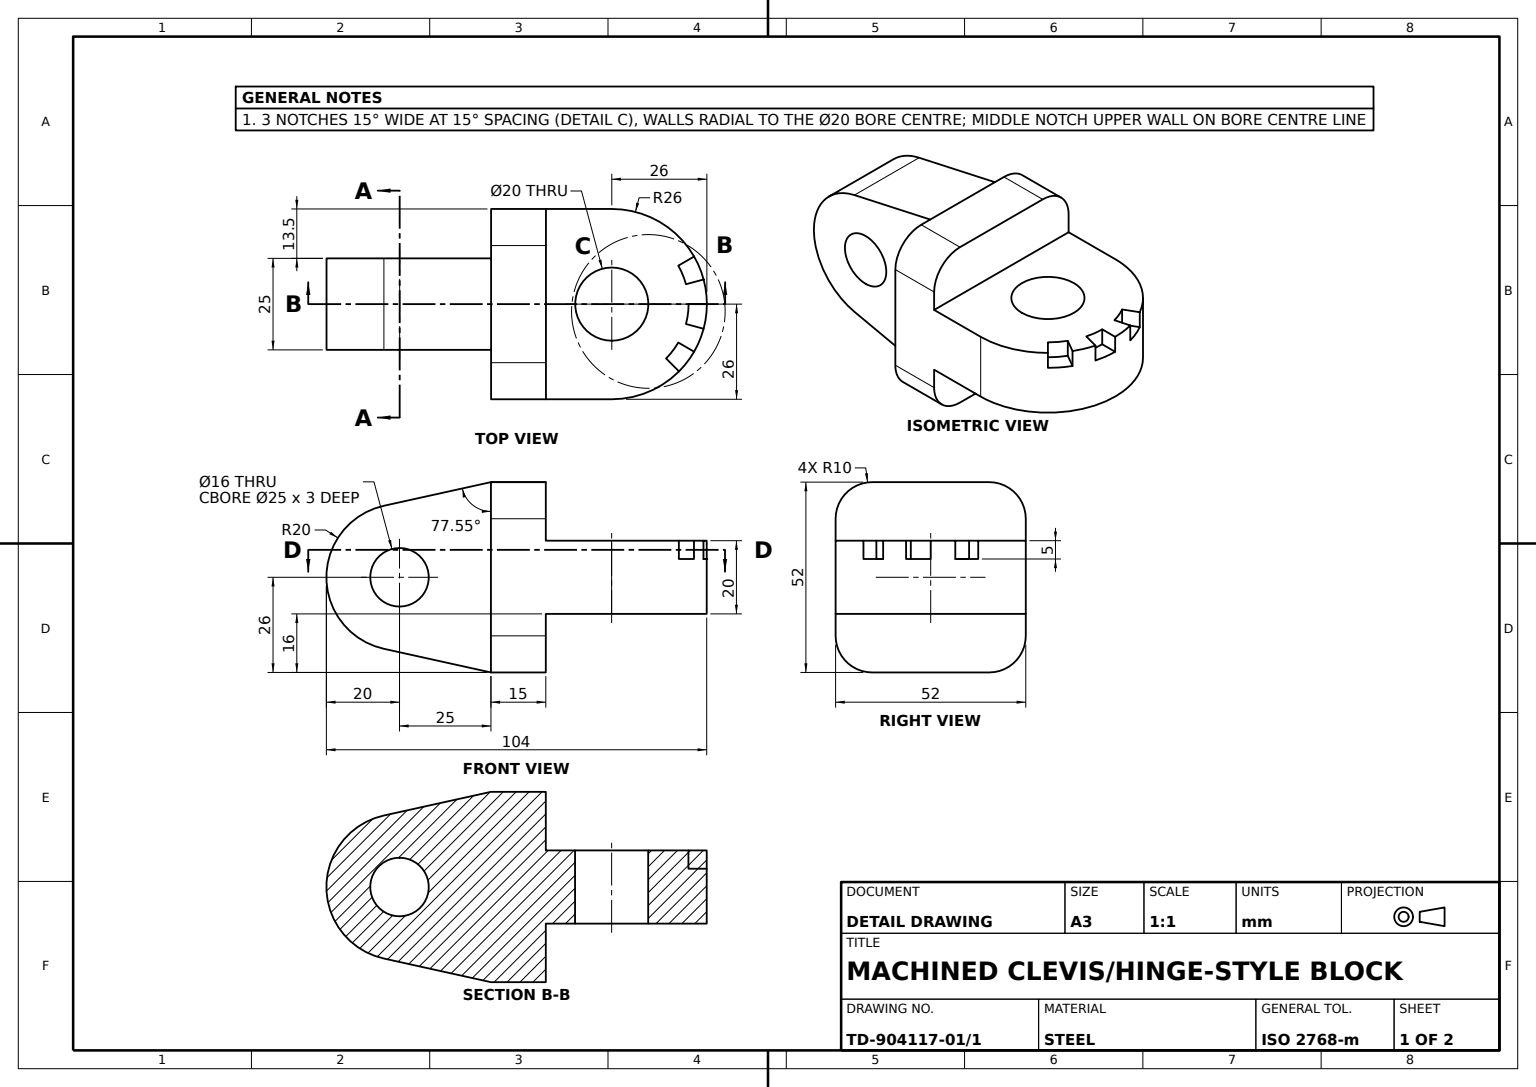
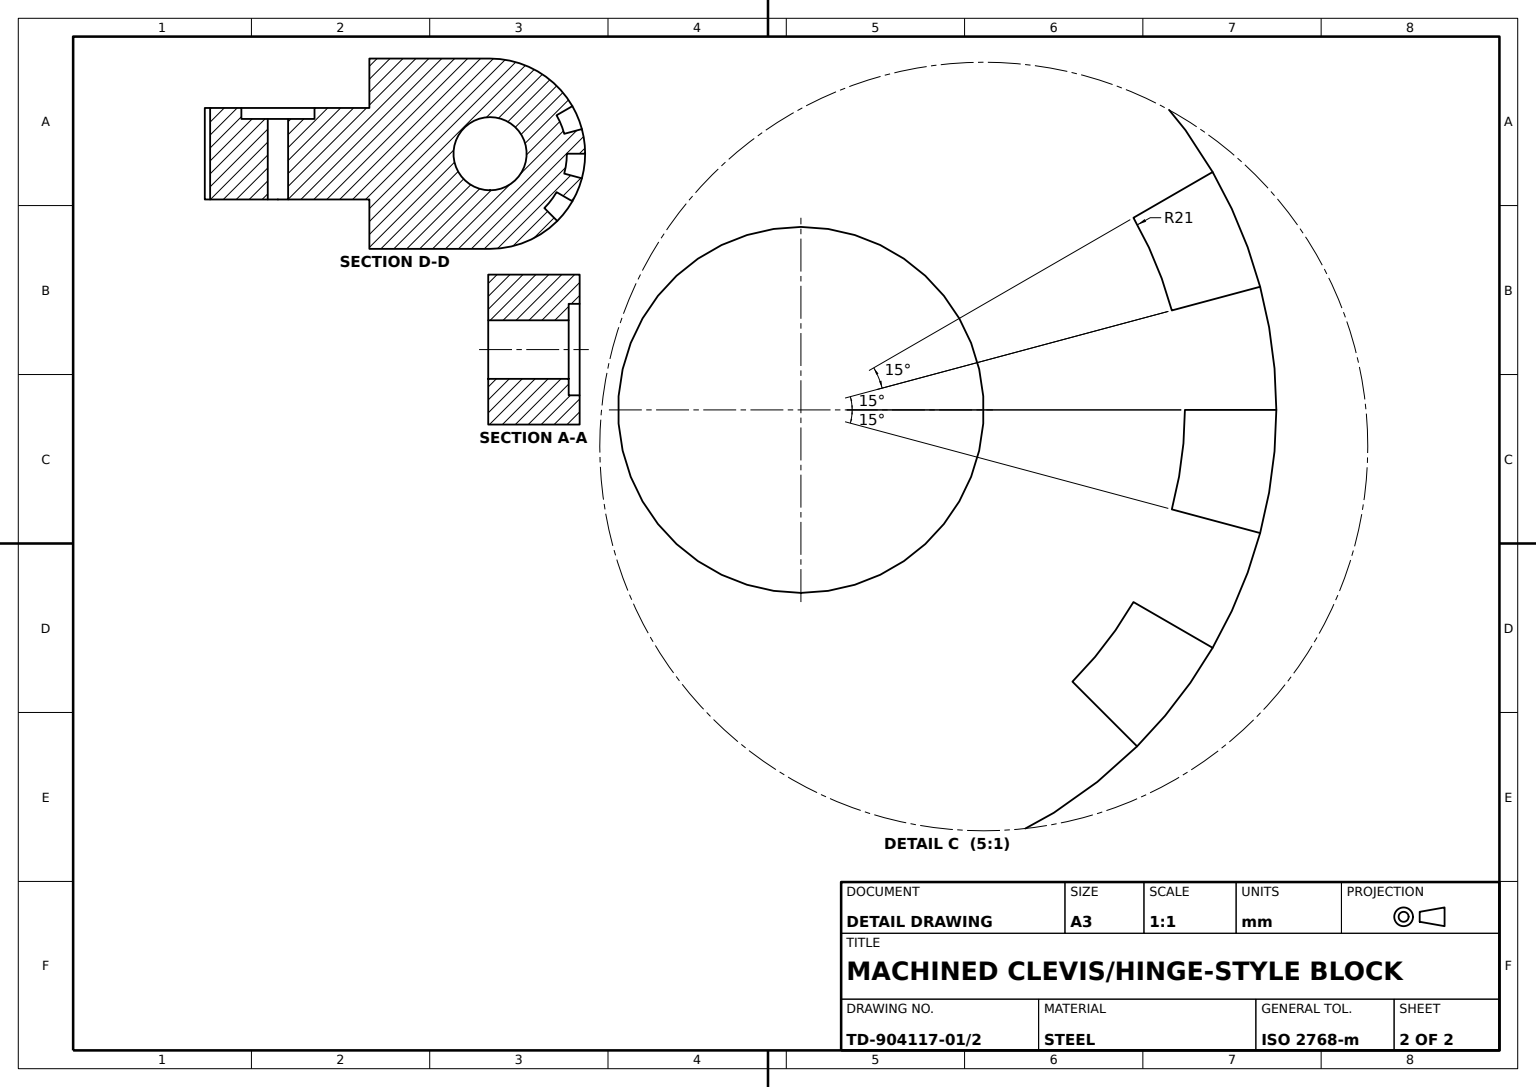
from build123d import *

# Parameters (mm, degrees)
ROUNDED_BASE_BLOCK_DEPTH   = 15
UPPER_BLOCK_DEPTH          = 52
UPPER_BLOCK_NOTCH_A_DEPTH  = 13.5
UPPER_START                = -13.5
UPPER_BLOCK_NOTCH_B_DEPTH  = 13.5
CROSS_BLOCK_DEPTH          = 52
CROSS_BLOCK_NOTCH_A_DEPTH  = 16
CROSS_START                = -16
CROSS_BLOCK_NOTCH_B_DEPTH  = 16
BORE_NOTCH_TEETH_CUT_DEPTH = 5
CROSS_BORE_10_SKETCH_R     = 10
CROSS_BORE_10_DEPTH        = 50
COUNTERBORE_25_SKETCH_R    = 12.5
COUNTERBORE_25_X3_DEPTH    = 3
MAIN_BORE_16_SKETCH_R      = 8
MAIN_BORE_16_DEPTH         = 50


with BuildPart() as part:
    # Base Block Profile Sketch → Rounded Base Block (new body)
    with BuildSketch(Plane.XY):
        with BuildLine():
            Line((-16, 0), (16, 0))
            ThreePointArc((16, 0), (23.071067812, 2.928932188), (26, 10))
            Line((26, 10), (26, 42))
            ThreePointArc((26, 42), (23.071067812, 49.071067812), (16, 52))
            Line((16, 52), (-16, 52))
            ThreePointArc((-16, 52), (-23.071067812, 49.071067812), (-26, 42))
            Line((-26, 42), (-26, 10))
            ThreePointArc((-26, 10), (-23.071067812, 2.928932188), (-16, 0))
        make_face()
    extrude(amount=ROUNDED_BASE_BLOCK_DEPTH)

    # Upper Block Profile Sketch → Upper Block (add)
    with BuildSketch(Plane.ZY.offset(26)):
        with BuildLine():
            Line((15, 52), (15, 0))
            Line((15, 0), (44.311040938, 6.470152944))
            ThreePointArc((44.311040938, 6.470152944), (60, 26), (44.311040938, 45.529847056))
            Line((44.311040938, 45.529847056), (15, 52))
        make_face()
    extrude(amount=-UPPER_BLOCK_DEPTH)

    # Upper Block Notch A Sketch → Upper Block Notch A (cut)
    with BuildSketch(Plane.ZY.offset(26)):
        with BuildLine():
            Line((15, 52), (44.311040938, 45.529847056))
            ThreePointArc((44.311040938, 45.529847056), (60, 26), (44.311040938, 6.470152944))
            Line((44.311040938, 6.470152944), (15, 0))
            Line((15, 0), (15, 52))
        make_face()
    extrude(amount=-UPPER_BLOCK_NOTCH_A_DEPTH, mode=Mode.SUBTRACT)

    # Upper Block Notch B Sketch → Upper Block Notch B (cut)
    with BuildSketch(Plane(origin=(26, 0, 0), x_dir=(0, 0, -1), z_dir=(1, 0, 0)).offset(UPPER_START)):
        with BuildLine():
            Line((-15, 52), (-15, 0))
            Line((-15, 0), (-44.311040938, 6.470152944))
            ThreePointArc((-44.311040938, 6.470152944), (-60, 26), (-44.311040938, 45.529847056))
            Line((-44.311040938, 45.529847056), (-15, 52))
        make_face()
    extrude(amount=UPPER_BLOCK_NOTCH_B_DEPTH, mode=Mode.SUBTRACT)

    # Cross Block Profile Sketch → Cross Block (add)
    with BuildSketch(Plane(origin=(0, 52, 0), x_dir=(1, 0, 0), z_dir=(0, 1, 0))):
        with BuildLine():
            Line((-26, 0), (-26, 18))
            ThreePointArc((-26, 18), (0, 44), (26, 18))
            Line((26, 18), (26, 0))
            Line((26, 0), (-26, 0))
        make_face()
    extrude(amount=-CROSS_BLOCK_DEPTH)

    # Cross Block Notch A Sketch → Cross Block Notch A (cut)
    with BuildSketch(Plane(origin=(0, 52, 0), x_dir=(1, 0, 0), z_dir=(0, 1, 0))):
        with BuildLine():
            Line((-26, 0), (26, 0))
            Line((26, 0), (26, 18))
            ThreePointArc((26, 18), (0, 44), (-26, 18))
            Line((-26, 18), (-26, 0))
        make_face()
    extrude(amount=-CROSS_BLOCK_NOTCH_A_DEPTH, mode=Mode.SUBTRACT)

    # Cross Block Notch B Sketch → Cross Block Notch B (cut)
    with BuildSketch(Plane.XZ.offset(CROSS_START)):
        with BuildLine():
            Line((-26, 0), (26, 0))
            Line((26, 0), (26, -18))
            ThreePointArc((26, -18), (0, -44), (-26, -18))
            Line((-26, -18), (-26, 0))
        make_face()
    extrude(amount=CROSS_BLOCK_NOTCH_B_DEPTH, mode=Mode.SUBTRACT)

    # Bore Notch Teeth Sketch → Bore Notch Teeth Cut (cut)
    with BuildSketch(Plane(origin=(0, 36, 0), x_dir=(1, 0, 0), z_dir=(0, 1, 0))):
        with BuildLine():
            Line((-5.435199947, 38.284442352), (-6.729295173, 43.114071484))
            ThreePointArc((-6.729295173, 43.114071484), (-9.949769241, 42.020867845), (-13, 40.516660498))
            Line((-13, 40.516660498), (-10.5, 36.186533479))
            ThreePointArc((-10.5, 36.186533479), (-8.03635208, 37.401470183), (-5.435199947, 38.284442352))
        make_face()
        with BuildLine():
            Line((0, 44), (0, 39))
            ThreePointArc((0, 39), (2.741050037, 38.820342089), (5.435199947, 38.284442352))
            Line((5.435199947, 38.284442352), (6.729295173, 43.114071484))
            ThreePointArc((6.729295173, 43.114071484), (3.393680998, 43.777566396), (0, 44))
        make_face()
        with BuildLine():
            ThreePointArc((18.384776311, 36.384776311), (15.827797154, 38.627186848), (13, 40.516660498))
            Line((13, 40.516660498), (10.5, 36.186533479))
            ThreePointArc((10.5, 36.186533479), (12.783990009, 34.660420146), (14.849242405, 32.849242405))
            Line((14.849242405, 32.849242405), (18.384776311, 36.384776311))
        make_face()
    extrude(amount=-BORE_NOTCH_TEETH_CUT_DEPTH, mode=Mode.SUBTRACT)

    # Cross Bore Ø10 Sketch → Cross Bore Ø10 (cut)
    with BuildSketch(Plane(origin=(0, 36, 0), x_dir=(1, 0, 0), z_dir=(0, 1, 0))):
        with Locations(Location((0, 18, 0), (0, 0, 180))):
            Circle(CROSS_BORE_10_SKETCH_R)
    extrude(amount=-CROSS_BORE_10_DEPTH, mode=Mode.SUBTRACT)

    # Counterbore Ø25 Sketch → Counterbore Ø25 x3 (cut)
    with BuildSketch(Plane.ZY.offset(12.5)):
        with Locations(Location((40, 26, 0), (0, 0, 270))):
            Circle(COUNTERBORE_25_SKETCH_R)
    extrude(amount=-COUNTERBORE_25_X3_DEPTH, mode=Mode.SUBTRACT)

    # Main Bore Ø16 Sketch → Main Bore Ø16 (cut)
    with BuildSketch(Plane.ZY.offset(9.5)):
        with Locations(Location((40, 26, 0), (0, 0, 270))):
            Circle(MAIN_BORE_16_SKETCH_R)
    extrude(amount=-MAIN_BORE_16_DEPTH, mode=Mode.SUBTRACT)


solid = part.part
